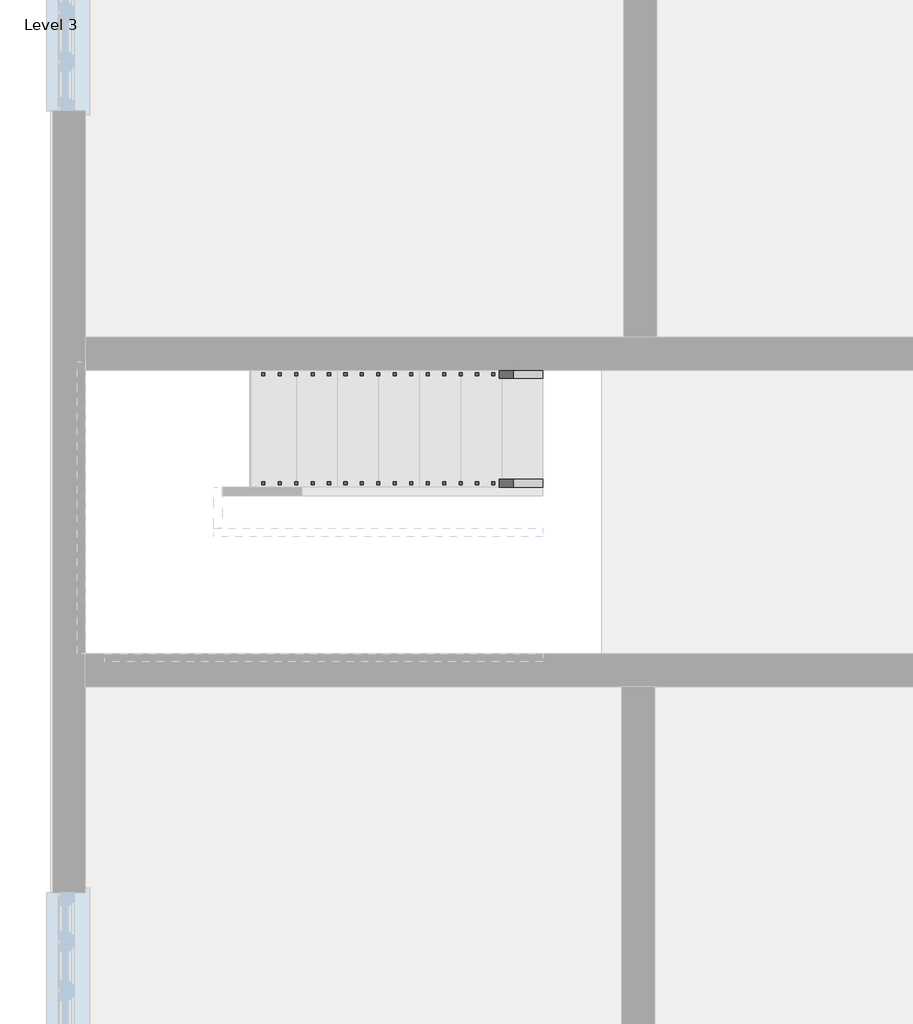
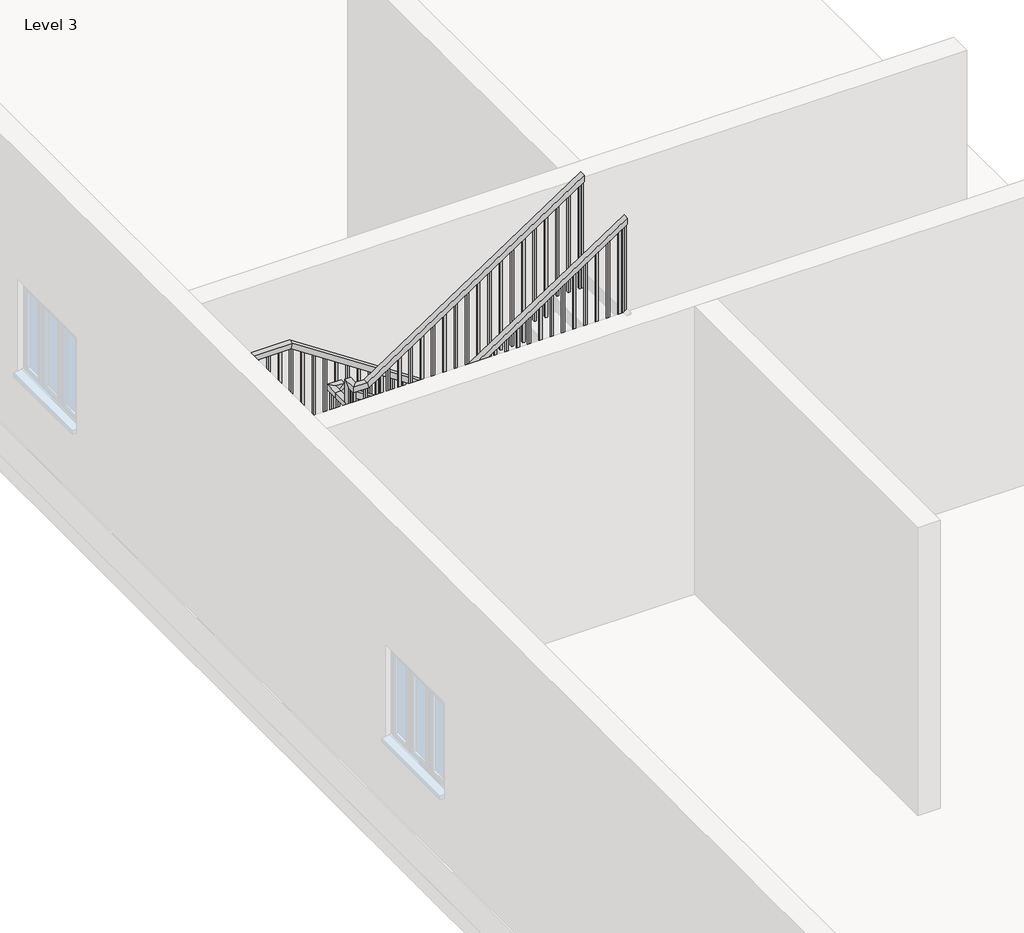
# One storey, part 2 of 3: 2 railings.
"""IFC4 building model written with IfcOpenShell, lengths in millimetres."""

from ifc_helpers import new_model, si_unit, frame, origin, place, context, project, spatial, polyline, outline, extrude, faceted_brep, element, save

model = new_model("IFC4")

# Units and contexts
model_context = context("Model", 3, world=origin())
ifc_project = project(units=[si_unit("LENGTHUNIT", "METRE", prefix="MILLI")], contexts=[model_context])

# Site, building, storey
site = spatial("IfcSite", under=ifc_project)
building = spatial("IfcBuilding", under=site)
storey = spatial("IfcBuildingStorey", under=building, Name="Level 3", Elevation=6096.0)

# Railings
placement = place(None, origin())
element("IfcRailing", 1, ObjectType="Handrail - Rectangular", at=placement, inside=storey, context=model_context, shape_type="SolidModel", body=[
    faceted_brep([(-2118.1728655, 1141.7797121, 7178.3222222), (-2118.1728655, 1141.7797121, 7117.4243166), (-2118.1728655, 1192.5797121, 7117.4243166), (-2118.1728655, 1192.5797121, 7178.3222222), (-4150.1728655, 1141.7797121, 8521.7), (-4165.4470084, 1141.7797121, 8470.9), (-4165.4470084, 1192.5797121, 8470.9), (-4150.1728655, 1192.5797121, 8521.7), (-4893.1394105, 1141.7797121, 8521.7), (-4893.1394105, 1141.7797121, 8470.9), (-4943.9394105, 1192.5797121, 8470.9), (-4943.9394105, 1192.5797121, 8521.7), (-4893.1394105, -509.2202879, 8521.7), (-4893.1394105, -509.2202879, 8470.9), (-4943.9394105, -560.0202879, 8470.9), (-4943.9394105, -560.0202879, 8521.7), (-4404.1728655, -509.2202879, 8521.7), (-4388.8987225, -509.2202879, 8470.9), (-4388.8987225, -560.0202879, 8470.9), (-4404.1728655, -560.0202879, 8521.7), (-2118.1728655, -509.2202879, 10033.0), (-2118.1728655, -560.0202879, 10033.0), (-2118.1728655, -560.0202879, 9972.1020944), (-2118.1728655, -509.2202879, 9972.1020944)], [[[0, 1, 2, 3]], [[1, 0, 4, 5]], [[2, 1, 5, 6]], [[3, 2, 6, 7]], [[0, 3, 7, 4]], [[5, 4, 8, 9]], [[6, 5, 9, 10]], [[7, 6, 10, 11]], [[4, 7, 11, 8]], [[9, 8, 12, 13]], [[10, 9, 13, 14]], [[11, 10, 14, 15]], [[8, 11, 15, 12]], [[13, 12, 16, 17]], [[14, 13, 17, 18]], [[15, 14, 18, 19]], [[12, 15, 19, 16]], [[20, 21, 22, 23]], [[17, 16, 20, 23]], [[18, 17, 23, 22]], [[19, 18, 22, 21]], [[16, 19, 21, 20]]]),
    extrude(outline(polyline([(9940.6057396, -2165.8144105), (9928.0115729, -2184.8644105), (8950.6777778, -2184.8644105), (8950.6777778, -2165.8144105), (9940.6057396, -2165.8144105)])), frame((0.0, -544.1452879, 0.0), z_axis=(0.0, 1.0, 0.0), x_axis=(0.0, 0.0, 1.0)), (0.0, 0.0, 1.0), 19.05),
    extrude(outline(polyline([(9873.4368507, -2267.4144105), (9860.842684, -2286.4644105), (8950.6777778, -2286.4644105), (8950.6777778, -2267.4144105), (9873.4368507, -2267.4144105)])), frame((0.0, -544.1452879, 0.0), z_axis=(0.0, 1.0, 0.0), x_axis=(0.0, 0.0, 1.0)), (0.0, 0.0, 1.0), 19.05),
    extrude(outline(polyline([(9806.2679618, -2369.0144105), (9793.6737951, -2388.0644105), (8782.7555556, -2388.0644105), (8782.7555556, -2369.0144105), (9806.2679618, -2369.0144105)])), frame((0.0, -544.1452879, 0.0), z_axis=(0.0, 1.0, 0.0), x_axis=(0.0, 0.0, 1.0)), (0.0, 0.0, 1.0), 19.05),
    extrude(outline(polyline([(9739.0990729, -2470.6144105), (9726.5049062, -2489.6644105), (8782.7555556, -2489.6644105), (8782.7555556, -2470.6144105), (9739.0990729, -2470.6144105)])), frame((0.0, -544.1452879, 0.0), z_axis=(0.0, 1.0, 0.0), x_axis=(0.0, 0.0, 1.0)), (0.0, 0.0, 1.0), 19.05),
    extrude(outline(polyline([(9671.930184, -2572.2144105), (9659.3360174, -2591.2644105), (8782.7555556, -2591.2644105), (8782.7555556, -2572.2144105), (9671.930184, -2572.2144105)])), frame((0.0, -544.1452879, 0.0), z_axis=(0.0, 1.0, 0.0), x_axis=(0.0, 0.0, 1.0)), (0.0, 0.0, 1.0), 19.05),
    extrude(outline(polyline([(9604.7612951, -2673.8144105), (9592.1671285, -2692.8644105), (8614.8333333, -2692.8644105), (8614.8333333, -2673.8144105), (9604.7612951, -2673.8144105)])), frame((0.0, -544.1452879, 0.0), z_axis=(0.0, 1.0, 0.0), x_axis=(0.0, 0.0, 1.0)), (0.0, 0.0, 1.0), 19.05),
    extrude(outline(polyline([(9537.5924062, -2775.4144105), (9524.9982396, -2794.4644105), (8614.8333333, -2794.4644105), (8614.8333333, -2775.4144105), (9537.5924062, -2775.4144105)])), frame((0.0, -544.1452879, 0.0), z_axis=(0.0, 1.0, 0.0), x_axis=(0.0, 0.0, 1.0)), (0.0, 0.0, 1.0), 19.05),
    extrude(outline(polyline([(9470.4235174, -2877.0144105), (9457.8293507, -2896.0644105), (8446.9111111, -2896.0644105), (8446.9111111, -2877.0144105), (9470.4235174, -2877.0144105)])), frame((0.0, -544.1452879, 0.0), z_axis=(0.0, 1.0, 0.0), x_axis=(0.0, 0.0, 1.0)), (0.0, 0.0, 1.0), 19.05),
    extrude(outline(polyline([(9403.2546285, -2978.6144105), (9390.6604618, -2997.6644105), (8446.9111111, -2997.6644105), (8446.9111111, -2978.6144105), (9403.2546285, -2978.6144105)])), frame((0.0, -544.1452879, 0.0), z_axis=(0.0, 1.0, 0.0), x_axis=(0.0, 0.0, 1.0)), (0.0, 0.0, 1.0), 19.05),
    extrude(outline(polyline([(9336.0857396, -3080.2144105), (9323.4915729, -3099.2644105), (8446.9111111, -3099.2644105), (8446.9111111, -3080.2144105), (9336.0857396, -3080.2144105)])), frame((0.0, -544.1452879, 0.0), z_axis=(0.0, 1.0, 0.0), x_axis=(0.0, 0.0, 1.0)), (0.0, 0.0, 1.0), 19.05),
    extrude(outline(polyline([(9268.9168507, -3181.8144105), (9256.322684, -3200.8644105), (8278.9888889, -3200.8644105), (8278.9888889, -3181.8144105), (9268.9168507, -3181.8144105)])), frame((0.0, -544.1452879, 0.0), z_axis=(0.0, 1.0, 0.0), x_axis=(0.0, 0.0, 1.0)), (0.0, 0.0, 1.0), 19.05),
    extrude(outline(polyline([(9201.7479618, -3283.4144105), (9189.1537951, -3302.4644105), (8278.9888889, -3302.4644105), (8278.9888889, -3283.4144105), (9201.7479618, -3283.4144105)])), frame((0.0, -544.1452879, 0.0), z_axis=(0.0, 1.0, 0.0), x_axis=(0.0, 0.0, 1.0)), (0.0, 0.0, 1.0), 19.05),
    extrude(outline(polyline([(9134.5790729, -3385.0144105), (9121.9849062, -3404.0644105), (8111.0666667, -3404.0644105), (8111.0666667, -3385.0144105), (9134.5790729, -3385.0144105)])), frame((0.0, -544.1452879, 0.0), z_axis=(0.0, 1.0, 0.0), x_axis=(0.0, 0.0, 1.0)), (0.0, 0.0, 1.0), 19.05),
    extrude(outline(polyline([(9067.410184, -3486.6144105), (9054.8160174, -3505.6644105), (8111.0666667, -3505.6644105), (8111.0666667, -3486.6144105), (9067.410184, -3486.6144105)])), frame((0.0, -544.1452879, 0.0), z_axis=(0.0, 1.0, 0.0), x_axis=(0.0, 0.0, 1.0)), (0.0, 0.0, 1.0), 19.05),
    extrude(outline(polyline([(9000.2412951, -3588.2144105), (8987.6471285, -3607.2644105), (8111.0666667, -3607.2644105), (8111.0666667, -3588.2144105), (9000.2412951, -3588.2144105)])), frame((0.0, -544.1452879, 0.0), z_axis=(0.0, 1.0, 0.0), x_axis=(0.0, 0.0, 1.0)), (0.0, 0.0, 1.0), 19.05),
    extrude(outline(polyline([(8933.0724062, -3689.8144105), (8920.4782396, -3708.8644105), (7943.1444444, -3708.8644105), (7943.1444444, -3689.8144105), (8933.0724062, -3689.8144105)])), frame((0.0, -544.1452879, 0.0), z_axis=(0.0, 1.0, 0.0), x_axis=(0.0, 0.0, 1.0)), (0.0, 0.0, 1.0), 19.05),
    extrude(outline(polyline([(8865.9035174, -3791.4144105), (8853.3093507, -3810.4644105), (7943.1444444, -3810.4644105), (7943.1444444, -3791.4144105), (8865.9035174, -3791.4144105)])), frame((0.0, -544.1452879, 0.0), z_axis=(0.0, 1.0, 0.0), x_axis=(0.0, 0.0, 1.0)), (0.0, 0.0, 1.0), 19.05),
    extrude(outline(polyline([(8798.7346285, -3893.0144105), (8786.1404618, -3912.0644105), (7775.2222222, -3912.0644105), (7775.2222222, -3893.0144105), (8798.7346285, -3893.0144105)])), frame((0.0, -544.1452879, 0.0), z_axis=(0.0, 1.0, 0.0), x_axis=(0.0, 0.0, 1.0)), (0.0, 0.0, 1.0), 19.05),
    extrude(outline(polyline([(8731.5657396, -3994.6144105), (8718.9715729, -4013.6644105), (7775.2222222, -4013.6644105), (7775.2222222, -3994.6144105), (8731.5657396, -3994.6144105)])), frame((0.0, -544.1452879, 0.0), z_axis=(0.0, 1.0, 0.0), x_axis=(0.0, 0.0, 1.0)), (0.0, 0.0, 1.0), 19.05),
    extrude(outline(polyline([(8664.3968507, -4096.2144105), (8651.802684, -4115.2644105), (7775.2222222, -4115.2644105), (7775.2222222, -4096.2144105), (8664.3968507, -4096.2144105)])), frame((0.0, -544.1452879, 0.0), z_axis=(0.0, 1.0, 0.0), x_axis=(0.0, 0.0, 1.0)), (0.0, 0.0, 1.0), 19.05),
    extrude(outline(polyline([(8597.2279618, -4197.8144105), (8584.6337951, -4216.8644105), (7607.3, -4216.8644105), (7607.3, -4197.8144105), (8597.2279618, -4197.8144105)])), frame((0.0, -544.1452879, 0.0), z_axis=(0.0, 1.0, 0.0), x_axis=(0.0, 0.0, 1.0)), (0.0, 0.0, 1.0), 19.05),
    extrude(outline(polyline([(8530.0590729, -4299.4144105), (8517.4649062, -4318.4644105), (7607.3, -4318.4644105), (7607.3, -4299.4144105), (8530.0590729, -4299.4144105)])), frame((0.0, -544.1452879, 0.0), z_axis=(0.0, 1.0, 0.0), x_axis=(0.0, 0.0, 1.0)), (0.0, 0.0, 1.0), 19.05),
    extrude(outline(polyline([(-4420.0644105, -544.1452879), (-4420.0644105, -525.0952879), (-4401.0144105, -525.0952879), (-4401.0144105, -544.1452879), (-4420.0644105, -544.1452879)])), frame((0.0, 0.0, 7607.3), z_axis=(0.0, 0.0, 1.0), x_axis=(1.0, 0.0, 0.0)), (0.0, 0.0, 1.0), 863.6),
    extrude(outline(polyline([(-4521.6644105, -544.1452879), (-4521.6644105, -525.0952879), (-4502.6144105, -525.0952879), (-4502.6144105, -544.1452879), (-4521.6644105, -544.1452879)])), frame((0.0, 0.0, 7607.3), z_axis=(0.0, 0.0, 1.0), x_axis=(1.0, 0.0, 0.0)), (0.0, 0.0, 1.0), 863.6),
    extrude(outline(polyline([(-4623.2644105, -544.1452879), (-4623.2644105, -525.0952879), (-4604.2144105, -525.0952879), (-4604.2144105, -544.1452879), (-4623.2644105, -544.1452879)])), frame((0.0, 0.0, 7607.3), z_axis=(0.0, 0.0, 1.0), x_axis=(1.0, 0.0, 0.0)), (0.0, 0.0, 1.0), 863.6),
    extrude(outline(polyline([(-4724.8644105, -544.1452879), (-4724.8644105, -525.0952879), (-4705.8144105, -525.0952879), (-4705.8144105, -544.1452879), (-4724.8644105, -544.1452879)])), frame((0.0, 0.0, 7607.3), z_axis=(0.0, 0.0, 1.0), x_axis=(1.0, 0.0, 0.0)), (0.0, 0.0, 1.0), 863.6),
    extrude(outline(polyline([(-4826.4644105, -544.1452879), (-4826.4644105, -525.0952879), (-4807.4144105, -525.0952879), (-4807.4144105, -544.1452879), (-4826.4644105, -544.1452879)])), frame((0.0, 0.0, 7607.3), z_axis=(0.0, 0.0, 1.0), x_axis=(1.0, 0.0, 0.0)), (0.0, 0.0, 1.0), 863.6),
    extrude(outline(polyline([(-4928.0644105, -448.8952879), (-4909.0144105, -448.8952879), (-4909.0144105, -467.9452879), (-4928.0644105, -467.9452879), (-4928.0644105, -448.8952879)])), frame((0.0, 0.0, 7607.3), z_axis=(0.0, 0.0, 1.0), x_axis=(1.0, 0.0, 0.0)), (0.0, 0.0, 1.0), 863.6),
    extrude(outline(polyline([(-4928.0644105, -347.2952879), (-4909.0144105, -347.2952879), (-4909.0144105, -366.3452879), (-4928.0644105, -366.3452879), (-4928.0644105, -347.2952879)])), frame((0.0, 0.0, 7607.3), z_axis=(0.0, 0.0, 1.0), x_axis=(1.0, 0.0, 0.0)), (0.0, 0.0, 1.0), 863.6),
    extrude(outline(polyline([(-4928.0644105, -245.6952879), (-4909.0144105, -245.6952879), (-4909.0144105, -264.7452879), (-4928.0644105, -264.7452879), (-4928.0644105, -245.6952879)])), frame((0.0, 0.0, 7607.3), z_axis=(0.0, 0.0, 1.0), x_axis=(1.0, 0.0, 0.0)), (0.0, 0.0, 1.0), 863.6),
    extrude(outline(polyline([(-4928.0644105, -144.0952879), (-4909.0144105, -144.0952879), (-4909.0144105, -163.1452879), (-4928.0644105, -163.1452879), (-4928.0644105, -144.0952879)])), frame((0.0, 0.0, 7607.3), z_axis=(0.0, 0.0, 1.0), x_axis=(1.0, 0.0, 0.0)), (0.0, 0.0, 1.0), 863.6),
    extrude(outline(polyline([(-4928.0644105, -42.4952879), (-4909.0144105, -42.4952879), (-4909.0144105, -61.5452879), (-4928.0644105, -61.5452879), (-4928.0644105, -42.4952879)])), frame((0.0, 0.0, 7607.3), z_axis=(0.0, 0.0, 1.0), x_axis=(1.0, 0.0, 0.0)), (0.0, 0.0, 1.0), 863.6),
    extrude(outline(polyline([(-4928.0644105, 59.1047121), (-4909.0144105, 59.1047121), (-4909.0144105, 40.0547121), (-4928.0644105, 40.0547121), (-4928.0644105, 59.1047121)])), frame((0.0, 0.0, 7607.3), z_axis=(0.0, 0.0, 1.0), x_axis=(1.0, 0.0, 0.0)), (0.0, 0.0, 1.0), 863.6),
    extrude(outline(polyline([(-4928.0644105, 160.7047121), (-4909.0144105, 160.7047121), (-4909.0144105, 141.6547121), (-4928.0644105, 141.6547121), (-4928.0644105, 160.7047121)])), frame((0.0, 0.0, 7607.3), z_axis=(0.0, 0.0, 1.0), x_axis=(1.0, 0.0, 0.0)), (0.0, 0.0, 1.0), 863.6),
    extrude(outline(polyline([(-4928.0644105, 262.3047121), (-4909.0144105, 262.3047121), (-4909.0144105, 243.2547121), (-4928.0644105, 243.2547121), (-4928.0644105, 262.3047121)])), frame((0.0, 0.0, 7607.3), z_axis=(0.0, 0.0, 1.0), x_axis=(1.0, 0.0, 0.0)), (0.0, 0.0, 1.0), 863.6),
    extrude(outline(polyline([(-4928.0644105, 363.9047121), (-4909.0144105, 363.9047121), (-4909.0144105, 344.8547121), (-4928.0644105, 344.8547121), (-4928.0644105, 363.9047121)])), frame((0.0, 0.0, 7607.3), z_axis=(0.0, 0.0, 1.0), x_axis=(1.0, 0.0, 0.0)), (0.0, 0.0, 1.0), 863.6),
    extrude(outline(polyline([(-4928.0644105, 465.5047121), (-4909.0144105, 465.5047121), (-4909.0144105, 446.4547121), (-4928.0644105, 446.4547121), (-4928.0644105, 465.5047121)])), frame((0.0, 0.0, 7607.3), z_axis=(0.0, 0.0, 1.0), x_axis=(1.0, 0.0, 0.0)), (0.0, 0.0, 1.0), 863.6),
    extrude(outline(polyline([(-4928.0644105, 567.1047121), (-4909.0144105, 567.1047121), (-4909.0144105, 548.0547121), (-4928.0644105, 548.0547121), (-4928.0644105, 567.1047121)])), frame((0.0, 0.0, 7607.3), z_axis=(0.0, 0.0, 1.0), x_axis=(1.0, 0.0, 0.0)), (0.0, 0.0, 1.0), 863.6),
    extrude(outline(polyline([(-4928.0644105, 668.7047121), (-4909.0144105, 668.7047121), (-4909.0144105, 649.6547121), (-4928.0644105, 649.6547121), (-4928.0644105, 668.7047121)])), frame((0.0, 0.0, 7607.3), z_axis=(0.0, 0.0, 1.0), x_axis=(1.0, 0.0, 0.0)), (0.0, 0.0, 1.0), 863.6),
    extrude(outline(polyline([(-4928.0644105, 770.3047121), (-4909.0144105, 770.3047121), (-4909.0144105, 751.2547121), (-4928.0644105, 751.2547121), (-4928.0644105, 770.3047121)])), frame((0.0, 0.0, 7607.3), z_axis=(0.0, 0.0, 1.0), x_axis=(1.0, 0.0, 0.0)), (0.0, 0.0, 1.0), 863.6),
    extrude(outline(polyline([(-4928.0644105, 871.9047121), (-4909.0144105, 871.9047121), (-4909.0144105, 852.8547121), (-4928.0644105, 852.8547121), (-4928.0644105, 871.9047121)])), frame((0.0, 0.0, 7607.3), z_axis=(0.0, 0.0, 1.0), x_axis=(1.0, 0.0, 0.0)), (0.0, 0.0, 1.0), 863.6),
    extrude(outline(polyline([(-4928.0644105, 973.5047121), (-4909.0144105, 973.5047121), (-4909.0144105, 954.4547121), (-4928.0644105, 954.4547121), (-4928.0644105, 973.5047121)])), frame((0.0, 0.0, 7607.3), z_axis=(0.0, 0.0, 1.0), x_axis=(1.0, 0.0, 0.0)), (0.0, 0.0, 1.0), 863.6),
    extrude(outline(polyline([(-4928.0644105, 1075.1047121), (-4909.0144105, 1075.1047121), (-4909.0144105, 1056.0547121), (-4928.0644105, 1056.0547121), (-4928.0644105, 1075.1047121)])), frame((0.0, 0.0, 7607.3), z_axis=(0.0, 0.0, 1.0), x_axis=(1.0, 0.0, 0.0)), (0.0, 0.0, 1.0), 863.6),
    extrude(outline(polyline([(-4851.8478655, 1176.7047121), (-4851.8478655, 1157.6547121), (-4870.8978655, 1157.6547121), (-4870.8978655, 1176.7047121), (-4851.8478655, 1176.7047121)])), frame((0.0, 0.0, 7607.3), z_axis=(0.0, 0.0, 1.0), x_axis=(1.0, 0.0, 0.0)), (0.0, 0.0, 1.0), 863.6),
    extrude(outline(polyline([(-4750.2478655, 1176.7047121), (-4750.2478655, 1157.6547121), (-4769.2978655, 1157.6547121), (-4769.2978655, 1176.7047121), (-4750.2478655, 1176.7047121)])), frame((0.0, 0.0, 7607.3), z_axis=(0.0, 0.0, 1.0), x_axis=(1.0, 0.0, 0.0)), (0.0, 0.0, 1.0), 863.6),
    extrude(outline(polyline([(-4648.6478655, 1176.7047121), (-4648.6478655, 1157.6547121), (-4667.6978655, 1157.6547121), (-4667.6978655, 1176.7047121), (-4648.6478655, 1176.7047121)])), frame((0.0, 0.0, 7607.3), z_axis=(0.0, 0.0, 1.0), x_axis=(1.0, 0.0, 0.0)), (0.0, 0.0, 1.0), 863.6),
    extrude(outline(polyline([(-4547.0478655, 1176.7047121), (-4547.0478655, 1157.6547121), (-4566.0978655, 1157.6547121), (-4566.0978655, 1176.7047121), (-4547.0478655, 1176.7047121)])), frame((0.0, 0.0, 7607.3), z_axis=(0.0, 0.0, 1.0), x_axis=(1.0, 0.0, 0.0)), (0.0, 0.0, 1.0), 863.6),
    extrude(outline(polyline([(-4445.4478655, 1176.7047121), (-4445.4478655, 1157.6547121), (-4464.4978655, 1157.6547121), (-4464.4978655, 1176.7047121), (-4445.4478655, 1176.7047121)])), frame((0.0, 0.0, 7607.3), z_axis=(0.0, 0.0, 1.0), x_axis=(1.0, 0.0, 0.0)), (0.0, 0.0, 1.0), 863.6),
    extrude(outline(polyline([(-4343.8478655, 1176.7047121), (-4343.8478655, 1157.6547121), (-4362.8978655, 1157.6547121), (-4362.8978655, 1176.7047121), (-4343.8478655, 1176.7047121)])), frame((0.0, 0.0, 7607.3), z_axis=(0.0, 0.0, 1.0), x_axis=(1.0, 0.0, 0.0)), (0.0, 0.0, 1.0), 863.6),
    extrude(outline(polyline([(-4242.2478655, 1176.7047121), (-4242.2478655, 1157.6547121), (-4261.2978655, 1157.6547121), (-4261.2978655, 1176.7047121), (-4242.2478655, 1176.7047121)])), frame((0.0, 0.0, 7607.3), z_axis=(0.0, 0.0, 1.0), x_axis=(1.0, 0.0, 0.0)), (0.0, 0.0, 1.0), 863.6),
    extrude(outline(polyline([(8454.505011, -4140.6478655), (8467.0991777, -4159.6978655), (7607.3, -4159.6978655), (7607.3, -4140.6478655), (8454.505011, -4140.6478655)])), frame((0.0, 1157.6547121, 0.0), z_axis=(0.0, 1.0, 0.0), x_axis=(0.0, 0.0, 1.0)), (0.0, 0.0, 1.0), 19.05),
    extrude(outline(polyline([(8387.3361222, -4039.0478655), (8399.9302888, -4058.0978655), (7439.3777778, -4058.0978655), (7439.3777778, -4039.0478655), (8387.3361222, -4039.0478655)])), frame((0.0, 1157.6547121, 0.0), z_axis=(0.0, 1.0, 0.0), x_axis=(0.0, 0.0, 1.0)), (0.0, 0.0, 1.0), 19.05),
    extrude(outline(polyline([(8320.1672333, -3937.4478655), (8332.7613999, -3956.4978655), (7439.3777778, -3956.4978655), (7439.3777778, -3937.4478655), (8320.1672333, -3937.4478655)])), frame((0.0, 1157.6547121, 0.0), z_axis=(0.0, 1.0, 0.0), x_axis=(0.0, 0.0, 1.0)), (0.0, 0.0, 1.0), 19.05),
    extrude(outline(polyline([(8252.9983444, -3835.8478655), (8265.592511, -3854.8978655), (7271.4555556, -3854.8978655), (7271.4555556, -3835.8478655), (8252.9983444, -3835.8478655)])), frame((0.0, 1157.6547121, 0.0), z_axis=(0.0, 1.0, 0.0), x_axis=(0.0, 0.0, 1.0)), (0.0, 0.0, 1.0), 19.05),
    extrude(outline(polyline([(8185.8294555, -3734.2478655), (8198.4236222, -3753.2978655), (7271.4555556, -3753.2978655), (7271.4555556, -3734.2478655), (8185.8294555, -3734.2478655)])), frame((0.0, 1157.6547121, 0.0), z_axis=(0.0, 1.0, 0.0), x_axis=(0.0, 0.0, 1.0)), (0.0, 0.0, 1.0), 19.05),
    extrude(outline(polyline([(8118.6605666, -3632.6478655), (8131.2547333, -3651.6978655), (7271.4555556, -3651.6978655), (7271.4555556, -3632.6478655), (8118.6605666, -3632.6478655)])), frame((0.0, 1157.6547121, 0.0), z_axis=(0.0, 1.0, 0.0), x_axis=(0.0, 0.0, 1.0)), (0.0, 0.0, 1.0), 19.05),
    extrude(outline(polyline([(8051.4916777, -3531.0478655), (8064.0858444, -3550.0978655), (7103.5333333, -3550.0978655), (7103.5333333, -3531.0478655), (8051.4916777, -3531.0478655)])), frame((0.0, 1157.6547121, 0.0), z_axis=(0.0, 1.0, 0.0), x_axis=(0.0, 0.0, 1.0)), (0.0, 0.0, 1.0), 19.05),
    extrude(outline(polyline([(7984.3227888, -3429.4478655), (7996.9169555, -3448.4978655), (7103.5333333, -3448.4978655), (7103.5333333, -3429.4478655), (7984.3227888, -3429.4478655)])), frame((0.0, 1157.6547121, 0.0), z_axis=(0.0, 1.0, 0.0), x_axis=(0.0, 0.0, 1.0)), (0.0, 0.0, 1.0), 19.05),
    extrude(outline(polyline([(7917.1538999, -3327.8478655), (7929.7480666, -3346.8978655), (6935.6111111, -3346.8978655), (6935.6111111, -3327.8478655), (7917.1538999, -3327.8478655)])), frame((0.0, 1157.6547121, 0.0), z_axis=(0.0, 1.0, 0.0), x_axis=(0.0, 0.0, 1.0)), (0.0, 0.0, 1.0), 19.05),
    extrude(outline(polyline([(7849.985011, -3226.2478655), (7862.5791777, -3245.2978655), (6935.6111111, -3245.2978655), (6935.6111111, -3226.2478655), (7849.985011, -3226.2478655)])), frame((0.0, 1157.6547121, 0.0), z_axis=(0.0, 1.0, 0.0), x_axis=(0.0, 0.0, 1.0)), (0.0, 0.0, 1.0), 19.05),
    extrude(outline(polyline([(7782.8161222, -3124.6478655), (7795.4102888, -3143.6978655), (6935.6111111, -3143.6978655), (6935.6111111, -3124.6478655), (7782.8161222, -3124.6478655)])), frame((0.0, 1157.6547121, 0.0), z_axis=(0.0, 1.0, 0.0), x_axis=(0.0, 0.0, 1.0)), (0.0, 0.0, 1.0), 19.05),
    extrude(outline(polyline([(7715.6472333, -3023.0478655), (7728.2413999, -3042.0978655), (6767.6888889, -3042.0978655), (6767.6888889, -3023.0478655), (7715.6472333, -3023.0478655)])), frame((0.0, 1157.6547121, 0.0), z_axis=(0.0, 1.0, 0.0), x_axis=(0.0, 0.0, 1.0)), (0.0, 0.0, 1.0), 19.05),
    extrude(outline(polyline([(7648.4783444, -2921.4478655), (7661.072511, -2940.4978655), (6767.6888889, -2940.4978655), (6767.6888889, -2921.4478655), (7648.4783444, -2921.4478655)])), frame((0.0, 1157.6547121, 0.0), z_axis=(0.0, 1.0, 0.0), x_axis=(0.0, 0.0, 1.0)), (0.0, 0.0, 1.0), 19.05),
    extrude(outline(polyline([(7581.3094555, -2819.8478655), (7593.9036222, -2838.8978655), (6599.7666667, -2838.8978655), (6599.7666667, -2819.8478655), (7581.3094555, -2819.8478655)])), frame((0.0, 1157.6547121, 0.0), z_axis=(0.0, 1.0, 0.0), x_axis=(0.0, 0.0, 1.0)), (0.0, 0.0, 1.0), 19.05),
    extrude(outline(polyline([(7514.1405666, -2718.2478655), (7526.7347333, -2737.2978655), (6599.7666667, -2737.2978655), (6599.7666667, -2718.2478655), (7514.1405666, -2718.2478655)])), frame((0.0, 1157.6547121, 0.0), z_axis=(0.0, 1.0, 0.0), x_axis=(0.0, 0.0, 1.0)), (0.0, 0.0, 1.0), 19.05),
    extrude(outline(polyline([(7446.9716777, -2616.6478655), (7459.5658444, -2635.6978655), (6599.7666667, -2635.6978655), (6599.7666667, -2616.6478655), (7446.9716777, -2616.6478655)])), frame((0.0, 1157.6547121, 0.0), z_axis=(0.0, 1.0, 0.0), x_axis=(0.0, 0.0, 1.0)), (0.0, 0.0, 1.0), 19.05),
    extrude(outline(polyline([(7379.8027888, -2515.0478655), (7392.3969555, -2534.0978655), (6431.8444444, -2534.0978655), (6431.8444444, -2515.0478655), (7379.8027888, -2515.0478655)])), frame((0.0, 1157.6547121, 0.0), z_axis=(0.0, 1.0, 0.0), x_axis=(0.0, 0.0, 1.0)), (0.0, 0.0, 1.0), 19.05),
    extrude(outline(polyline([(7312.6338999, -2413.4478655), (7325.2280666, -2432.4978655), (6431.8444444, -2432.4978655), (6431.8444444, -2413.4478655), (7312.6338999, -2413.4478655)])), frame((0.0, 1157.6547121, 0.0), z_axis=(0.0, 1.0, 0.0), x_axis=(0.0, 0.0, 1.0)), (0.0, 0.0, 1.0), 19.05),
    extrude(outline(polyline([(7245.465011, -2311.8478655), (7258.0591777, -2330.8978655), (6263.9222222, -2330.8978655), (6263.9222222, -2311.8478655), (7245.465011, -2311.8478655)])), frame((0.0, 1157.6547121, 0.0), z_axis=(0.0, 1.0, 0.0), x_axis=(0.0, 0.0, 1.0)), (0.0, 0.0, 1.0), 19.05),
    extrude(outline(polyline([(7178.2961222, -2210.2478655), (7190.8902888, -2229.2978655), (6263.9222222, -2229.2978655), (6263.9222222, -2210.2478655), (7178.2961222, -2210.2478655)])), frame((0.0, 1157.6547121, 0.0), z_axis=(0.0, 1.0, 0.0), x_axis=(0.0, 0.0, 1.0)), (0.0, 0.0, 1.0), 19.05),
    extrude(outline(polyline([(-4928.0644105, -525.0952879), (-4909.0144105, -525.0952879), (-4909.0144105, -544.1452879), (-4928.0644105, -544.1452879), (-4928.0644105, -525.0952879)])), frame((0.0, 0.0, 7607.3), z_axis=(0.0, 0.0, 1.0), x_axis=(1.0, 0.0, 0.0)), (0.0, 0.0, 1.0), 863.6),
    extrude(outline(polyline([(-4909.0144105, 1176.7047121), (-4909.0144105, 1157.6547121), (-4928.0644105, 1157.6547121), (-4928.0644105, 1176.7047121), (-4909.0144105, 1176.7047121)])), frame((0.0, 0.0, 7607.3), z_axis=(0.0, 0.0, 1.0), x_axis=(1.0, 0.0, 0.0)), (0.0, 0.0, 1.0), 863.6),
    extrude(outline(polyline([(9972.1020944, -2118.1728655), (9959.5079277, -2137.2228655), (8950.6777778, -2137.2228655), (8950.6777778, -2118.1728655), (9972.1020944, -2118.1728655)])), frame((0.0, -544.1452879, 0.0), z_axis=(0.0, 1.0, 0.0), x_axis=(0.0, 0.0, 1.0)), (0.0, 0.0, 1.0), 19.05),
    extrude(outline(polyline([(7117.4243166, -2118.1728655), (7130.0184833, -2137.2228655), (6263.9222222, -2137.2228655), (6263.9222222, -2118.1728655), (7117.4243166, -2118.1728655)])), frame((0.0, 1157.6547121, 0.0), z_axis=(0.0, 1.0, 0.0), x_axis=(0.0, 0.0, 1.0)), (0.0, 0.0, 1.0), 19.05),
])
element("IfcRailing", 2, ObjectType="Handrail - Rectangular", at=placement, inside=storey, context=model_context, shape_type="SolidModel", body=[
    faceted_brep([(-2118.1728655, 468.6797121, 7178.3222222), (-2118.1728655, 468.6797121, 7117.4243166), (-2118.1728655, 519.4797121, 7117.4243166), (-2118.1728655, 519.4797121, 7178.3222222), (-4073.9728655, 468.6797121, 8471.3233333), (-4124.7728655, 468.6797121, 8444.0098722), (-4124.7728655, 519.4797121, 8444.0098722), (-4073.9728655, 519.4797121, 8471.3233333), (-4073.9728655, 468.6797121, 8521.7), (-4124.7728655, 468.6797121, 8470.9), (-4124.7728655, 519.4797121, 8470.9), (-4073.9728655, 519.4797121, 8521.7), (-4150.1728655, 468.6797121, 8521.7), (-4150.1728655, 468.6797121, 8470.9), (-4200.9728655, 519.4797121, 8470.9), (-4200.9728655, 519.4797121, 8521.7), (-4150.1728655, 392.4797121, 8521.7), (-4150.1728655, 392.4797121, 8470.9), (-4200.9728655, 392.4797121, 8470.9), (-4200.9728655, 392.4797121, 8521.7), (-4150.1728655, 240.0797121, 8521.7), (-4150.1728655, 189.2797121, 8470.9), (-4200.9728655, 189.2797121, 8470.9), (-4200.9728655, 240.0797121, 8521.7), (-4150.1728655, 240.0797121, 8739.9988889), (-4150.1728655, 189.2797121, 8689.1988889), (-4200.9728655, 189.2797121, 8689.1988889), (-4200.9728655, 240.0797121, 8739.9988889), (-4150.1728655, 163.8797121, 8739.9988889), (-4150.1728655, 163.8797121, 8689.1988889), (-4200.9728655, 113.0797121, 8689.1988889), (-4200.9728655, 113.0797121, 8739.9988889), (-4073.9728655, 163.8797121, 8739.9988889), (-4058.6987225, 163.8797121, 8689.1988889), (-4058.6987225, 113.0797121, 8689.1988889), (-4073.9728655, 113.0797121, 8739.9988889), (-2118.1728655, 163.8797121, 10033.0), (-2118.1728655, 113.0797121, 10033.0), (-2118.1728655, 113.0797121, 9972.1020944), (-2118.1728655, 163.8797121, 9972.1020944)], [[[0, 1, 2, 3]], [[1, 0, 4, 5]], [[2, 1, 5, 6]], [[3, 2, 6, 7]], [[0, 3, 7, 4]], [[5, 4, 8, 9]], [[6, 5, 9, 10]], [[7, 6, 10, 11]], [[4, 7, 11, 8]], [[9, 8, 12, 13]], [[10, 9, 13, 14]], [[11, 10, 14, 15]], [[8, 11, 15, 12]], [[13, 12, 16, 17]], [[14, 13, 17, 18]], [[15, 14, 18, 19]], [[12, 15, 19, 16]], [[17, 16, 20, 21]], [[18, 17, 21, 22]], [[19, 18, 22, 23]], [[16, 19, 23, 20]], [[21, 20, 24, 25]], [[22, 21, 25, 26]], [[23, 22, 26, 27]], [[20, 23, 27, 24]], [[25, 24, 28, 29]], [[26, 25, 29, 30]], [[27, 26, 30, 31]], [[24, 27, 31, 28]], [[29, 28, 32, 33]], [[30, 29, 33, 34]], [[31, 30, 34, 35]], [[28, 31, 35, 32]], [[36, 37, 38, 39]], [[33, 32, 36, 39]], [[34, 33, 39, 38]], [[35, 34, 38, 37]], [[32, 35, 37, 36]]]),
    extrude(outline(polyline([(9949.0127888, -2153.0978655), (8950.6777778, -2153.0978655), (8950.6777778, -2134.0478655), (9961.6069555, -2134.0478655), (9949.0127888, -2153.0978655)])), frame((0.0, 128.9547121, 0.0), z_axis=(0.0, 1.0, 0.0), x_axis=(0.0, 0.0, 1.0)), (0.0, 0.0, 1.0), 19.05),
    extrude(outline(polyline([(9881.8438999, -2254.6978655), (8950.6777778, -2254.6978655), (8950.6777778, -2235.6478655), (9894.4380666, -2235.6478655), (9881.8438999, -2254.6978655)])), frame((0.0, 128.9547121, 0.0), z_axis=(0.0, 1.0, 0.0), x_axis=(0.0, 0.0, 1.0)), (0.0, 0.0, 1.0), 19.05),
    extrude(outline(polyline([(9814.675011, -2356.2978655), (8950.6777778, -2356.2978655), (8950.6777778, -2337.2478655), (9827.2691777, -2337.2478655), (9814.675011, -2356.2978655)])), frame((0.0, 128.9547121, 0.0), z_axis=(0.0, 1.0, 0.0), x_axis=(0.0, 0.0, 1.0)), (0.0, 0.0, 1.0), 19.05),
    extrude(outline(polyline([(9747.5061222, -2457.8978655), (8782.7555556, -2457.8978655), (8782.7555556, -2438.8478655), (9760.1002888, -2438.8478655), (9747.5061222, -2457.8978655)])), frame((0.0, 128.9547121, 0.0), z_axis=(0.0, 1.0, 0.0), x_axis=(0.0, 0.0, 1.0)), (0.0, 0.0, 1.0), 19.05),
    extrude(outline(polyline([(9680.3372333, -2559.4978655), (8782.7555556, -2559.4978655), (8782.7555556, -2540.4478655), (9692.9313999, -2540.4478655), (9680.3372333, -2559.4978655)])), frame((0.0, 128.9547121, 0.0), z_axis=(0.0, 1.0, 0.0), x_axis=(0.0, 0.0, 1.0)), (0.0, 0.0, 1.0), 19.05),
    extrude(outline(polyline([(9613.1683444, -2661.0978655), (8614.8333333, -2661.0978655), (8614.8333333, -2642.0478655), (9625.762511, -2642.0478655), (9613.1683444, -2661.0978655)])), frame((0.0, 128.9547121, 0.0), z_axis=(0.0, 1.0, 0.0), x_axis=(0.0, 0.0, 1.0)), (0.0, 0.0, 1.0), 19.05),
    extrude(outline(polyline([(9545.9994555, -2762.6978655), (8614.8333333, -2762.6978655), (8614.8333333, -2743.6478655), (9558.5936222, -2743.6478655), (9545.9994555, -2762.6978655)])), frame((0.0, 128.9547121, 0.0), z_axis=(0.0, 1.0, 0.0), x_axis=(0.0, 0.0, 1.0)), (0.0, 0.0, 1.0), 19.05),
    extrude(outline(polyline([(9478.8305666, -2864.2978655), (8614.8333333, -2864.2978655), (8614.8333333, -2845.2478655), (9491.4247333, -2845.2478655), (9478.8305666, -2864.2978655)])), frame((0.0, 128.9547121, 0.0), z_axis=(0.0, 1.0, 0.0), x_axis=(0.0, 0.0, 1.0)), (0.0, 0.0, 1.0), 19.05),
    extrude(outline(polyline([(9411.6616777, -2965.8978655), (8446.9111111, -2965.8978655), (8446.9111111, -2946.8478655), (9424.2558444, -2946.8478655), (9411.6616777, -2965.8978655)])), frame((0.0, 128.9547121, 0.0), z_axis=(0.0, 1.0, 0.0), x_axis=(0.0, 0.0, 1.0)), (0.0, 0.0, 1.0), 19.05),
    extrude(outline(polyline([(9344.4927888, -3067.4978655), (8446.9111111, -3067.4978655), (8446.9111111, -3048.4478655), (9357.0869555, -3048.4478655), (9344.4927888, -3067.4978655)])), frame((0.0, 128.9547121, 0.0), z_axis=(0.0, 1.0, 0.0), x_axis=(0.0, 0.0, 1.0)), (0.0, 0.0, 1.0), 19.05),
    extrude(outline(polyline([(9277.3238999, -3169.0978655), (8278.9888889, -3169.0978655), (8278.9888889, -3150.0478655), (9289.9180666, -3150.0478655), (9277.3238999, -3169.0978655)])), frame((0.0, 128.9547121, 0.0), z_axis=(0.0, 1.0, 0.0), x_axis=(0.0, 0.0, 1.0)), (0.0, 0.0, 1.0), 19.05),
    extrude(outline(polyline([(9210.155011, -3270.6978655), (8278.9888889, -3270.6978655), (8278.9888889, -3251.6478655), (9222.7491777, -3251.6478655), (9210.155011, -3270.6978655)])), frame((0.0, 128.9547121, 0.0), z_axis=(0.0, 1.0, 0.0), x_axis=(0.0, 0.0, 1.0)), (0.0, 0.0, 1.0), 19.05),
    extrude(outline(polyline([(9142.9861222, -3372.2978655), (8278.9888889, -3372.2978655), (8278.9888889, -3353.2478655), (9155.5802888, -3353.2478655), (9142.9861222, -3372.2978655)])), frame((0.0, 128.9547121, 0.0), z_axis=(0.0, 1.0, 0.0), x_axis=(0.0, 0.0, 1.0)), (0.0, 0.0, 1.0), 19.05),
    extrude(outline(polyline([(9075.8172333, -3473.8978655), (8111.0666667, -3473.8978655), (8111.0666667, -3454.8478655), (9088.4113999, -3454.8478655), (9075.8172333, -3473.8978655)])), frame((0.0, 128.9547121, 0.0), z_axis=(0.0, 1.0, 0.0), x_axis=(0.0, 0.0, 1.0)), (0.0, 0.0, 1.0), 19.05),
    extrude(outline(polyline([(9008.6483444, -3575.4978655), (8111.0666667, -3575.4978655), (8111.0666667, -3556.4478655), (9021.242511, -3556.4478655), (9008.6483444, -3575.4978655)])), frame((0.0, 128.9547121, 0.0), z_axis=(0.0, 1.0, 0.0), x_axis=(0.0, 0.0, 1.0)), (0.0, 0.0, 1.0), 19.05),
    extrude(outline(polyline([(8941.4794555, -3677.0978655), (7943.1444444, -3677.0978655), (7943.1444444, -3658.0478655), (8954.0736222, -3658.0478655), (8941.4794555, -3677.0978655)])), frame((0.0, 128.9547121, 0.0), z_axis=(0.0, 1.0, 0.0), x_axis=(0.0, 0.0, 1.0)), (0.0, 0.0, 1.0), 19.05),
    extrude(outline(polyline([(8874.3105666, -3778.6978655), (7943.1444444, -3778.6978655), (7943.1444444, -3759.6478655), (8886.9047333, -3759.6478655), (8874.3105666, -3778.6978655)])), frame((0.0, 128.9547121, 0.0), z_axis=(0.0, 1.0, 0.0), x_axis=(0.0, 0.0, 1.0)), (0.0, 0.0, 1.0), 19.05),
    extrude(outline(polyline([(8807.1416777, -3880.2978655), (7943.1444444, -3880.2978655), (7943.1444444, -3861.2478655), (8819.7358444, -3861.2478655), (8807.1416777, -3880.2978655)])), frame((0.0, 128.9547121, 0.0), z_axis=(0.0, 1.0, 0.0), x_axis=(0.0, 0.0, 1.0)), (0.0, 0.0, 1.0), 19.05),
    extrude(outline(polyline([(8739.9727888, -3981.8978655), (7775.2222222, -3981.8978655), (7775.2222222, -3962.8478655), (8752.5669555, -3962.8478655), (8739.9727888, -3981.8978655)])), frame((0.0, 128.9547121, 0.0), z_axis=(0.0, 1.0, 0.0), x_axis=(0.0, 0.0, 1.0)), (0.0, 0.0, 1.0), 19.05),
    extrude(outline(polyline([(8672.8038999, -4083.4978655), (7775.2222222, -4083.4978655), (7775.2222222, -4064.4478655), (8685.3980666, -4064.4478655), (8672.8038999, -4083.4978655)])), frame((0.0, 128.9547121, 0.0), z_axis=(0.0, 1.0, 0.0), x_axis=(0.0, 0.0, 1.0)), (0.0, 0.0, 1.0), 19.05),
    extrude(outline(polyline([(-4166.0478655, 198.8047121), (-4166.0478655, 179.7547121), (-4185.0978655, 179.7547121), (-4185.0978655, 198.8047121), (-4166.0478655, 198.8047121)])), frame((0.0, 0.0, 7607.3), z_axis=(0.0, 0.0, 1.0), x_axis=(1.0, 0.0, 0.0)), (0.0, 0.0, 1.0), 1081.8988889),
    extrude(outline(polyline([(-4166.0478655, 300.4047121), (-4166.0478655, 281.3547121), (-4185.0978655, 281.3547121), (-4185.0978655, 300.4047121), (-4166.0478655, 300.4047121)])), frame((0.0, 0.0, 7607.3), z_axis=(0.0, 0.0, 1.0), x_axis=(1.0, 0.0, 0.0)), (0.0, 0.0, 1.0), 863.6),
    extrude(outline(polyline([(-4166.0478655, 402.0047121), (-4166.0478655, 382.9547121), (-4185.0978655, 382.9547121), (-4185.0978655, 402.0047121), (-4166.0478655, 402.0047121)])), frame((0.0, 0.0, 7607.3), z_axis=(0.0, 0.0, 1.0), x_axis=(1.0, 0.0, 0.0)), (0.0, 0.0, 1.0), 863.6),
    extrude(outline(polyline([(-4140.6478655, 484.5547121), (-4159.6978655, 484.5547121), (-4159.6978655, 503.6047121), (-4140.6478655, 503.6047121), (-4140.6478655, 484.5547121)])), frame((0.0, 0.0, 7607.3), z_axis=(0.0, 0.0, 1.0), x_axis=(1.0, 0.0, 0.0)), (0.0, 0.0, 1.0), 863.6),
    extrude(outline(polyline([(8399.9302888, -4058.0978655), (7439.3777778, -4058.0978655), (7439.3777778, -4039.0478655), (8387.3361222, -4039.0478655), (8399.9302888, -4058.0978655)])), frame((0.0, 484.5547121, 0.0), z_axis=(0.0, 1.0, 0.0), x_axis=(0.0, 0.0, 1.0)), (0.0, 0.0, 1.0), 19.05),
    extrude(outline(polyline([(8332.7613999, -3956.4978655), (7439.3777778, -3956.4978655), (7439.3777778, -3937.4478655), (8320.1672333, -3937.4478655), (8332.7613999, -3956.4978655)])), frame((0.0, 484.5547121, 0.0), z_axis=(0.0, 1.0, 0.0), x_axis=(0.0, 0.0, 1.0)), (0.0, 0.0, 1.0), 19.05),
    extrude(outline(polyline([(8265.592511, -3854.8978655), (7271.4555556, -3854.8978655), (7271.4555556, -3835.8478655), (8252.9983444, -3835.8478655), (8265.592511, -3854.8978655)])), frame((0.0, 484.5547121, 0.0), z_axis=(0.0, 1.0, 0.0), x_axis=(0.0, 0.0, 1.0)), (0.0, 0.0, 1.0), 19.05),
    extrude(outline(polyline([(8198.4236222, -3753.2978655), (7271.4555556, -3753.2978655), (7271.4555556, -3734.2478655), (8185.8294555, -3734.2478655), (8198.4236222, -3753.2978655)])), frame((0.0, 484.5547121, 0.0), z_axis=(0.0, 1.0, 0.0), x_axis=(0.0, 0.0, 1.0)), (0.0, 0.0, 1.0), 19.05),
    extrude(outline(polyline([(8131.2547333, -3651.6978655), (7271.4555556, -3651.6978655), (7271.4555556, -3632.6478655), (8118.6605666, -3632.6478655), (8131.2547333, -3651.6978655)])), frame((0.0, 484.5547121, 0.0), z_axis=(0.0, 1.0, 0.0), x_axis=(0.0, 0.0, 1.0)), (0.0, 0.0, 1.0), 19.05),
    extrude(outline(polyline([(8064.0858444, -3550.0978655), (7103.5333333, -3550.0978655), (7103.5333333, -3531.0478655), (8051.4916777, -3531.0478655), (8064.0858444, -3550.0978655)])), frame((0.0, 484.5547121, 0.0), z_axis=(0.0, 1.0, 0.0), x_axis=(0.0, 0.0, 1.0)), (0.0, 0.0, 1.0), 19.05),
    extrude(outline(polyline([(7996.9169555, -3448.4978655), (7103.5333333, -3448.4978655), (7103.5333333, -3429.4478655), (7984.3227888, -3429.4478655), (7996.9169555, -3448.4978655)])), frame((0.0, 484.5547121, 0.0), z_axis=(0.0, 1.0, 0.0), x_axis=(0.0, 0.0, 1.0)), (0.0, 0.0, 1.0), 19.05),
    extrude(outline(polyline([(7929.7480666, -3346.8978655), (6935.6111111, -3346.8978655), (6935.6111111, -3327.8478655), (7917.1538999, -3327.8478655), (7929.7480666, -3346.8978655)])), frame((0.0, 484.5547121, 0.0), z_axis=(0.0, 1.0, 0.0), x_axis=(0.0, 0.0, 1.0)), (0.0, 0.0, 1.0), 19.05),
    extrude(outline(polyline([(7862.5791777, -3245.2978655), (6935.6111111, -3245.2978655), (6935.6111111, -3226.2478655), (7849.985011, -3226.2478655), (7862.5791777, -3245.2978655)])), frame((0.0, 484.5547121, 0.0), z_axis=(0.0, 1.0, 0.0), x_axis=(0.0, 0.0, 1.0)), (0.0, 0.0, 1.0), 19.05),
    extrude(outline(polyline([(7795.4102888, -3143.6978655), (6935.6111111, -3143.6978655), (6935.6111111, -3124.6478655), (7782.8161222, -3124.6478655), (7795.4102888, -3143.6978655)])), frame((0.0, 484.5547121, 0.0), z_axis=(0.0, 1.0, 0.0), x_axis=(0.0, 0.0, 1.0)), (0.0, 0.0, 1.0), 19.05),
    extrude(outline(polyline([(7728.2413999, -3042.0978655), (6767.6888889, -3042.0978655), (6767.6888889, -3023.0478655), (7715.6472333, -3023.0478655), (7728.2413999, -3042.0978655)])), frame((0.0, 484.5547121, 0.0), z_axis=(0.0, 1.0, 0.0), x_axis=(0.0, 0.0, 1.0)), (0.0, 0.0, 1.0), 19.05),
    extrude(outline(polyline([(7661.072511, -2940.4978655), (6767.6888889, -2940.4978655), (6767.6888889, -2921.4478655), (7648.4783444, -2921.4478655), (7661.072511, -2940.4978655)])), frame((0.0, 484.5547121, 0.0), z_axis=(0.0, 1.0, 0.0), x_axis=(0.0, 0.0, 1.0)), (0.0, 0.0, 1.0), 19.05),
    extrude(outline(polyline([(7593.9036222, -2838.8978655), (6599.7666667, -2838.8978655), (6599.7666667, -2819.8478655), (7581.3094555, -2819.8478655), (7593.9036222, -2838.8978655)])), frame((0.0, 484.5547121, 0.0), z_axis=(0.0, 1.0, 0.0), x_axis=(0.0, 0.0, 1.0)), (0.0, 0.0, 1.0), 19.05),
    extrude(outline(polyline([(7526.7347333, -2737.2978655), (6599.7666667, -2737.2978655), (6599.7666667, -2718.2478655), (7514.1405666, -2718.2478655), (7526.7347333, -2737.2978655)])), frame((0.0, 484.5547121, 0.0), z_axis=(0.0, 1.0, 0.0), x_axis=(0.0, 0.0, 1.0)), (0.0, 0.0, 1.0), 19.05),
    extrude(outline(polyline([(7459.5658444, -2635.6978655), (6599.7666667, -2635.6978655), (6599.7666667, -2616.6478655), (7446.9716777, -2616.6478655), (7459.5658444, -2635.6978655)])), frame((0.0, 484.5547121, 0.0), z_axis=(0.0, 1.0, 0.0), x_axis=(0.0, 0.0, 1.0)), (0.0, 0.0, 1.0), 19.05),
    extrude(outline(polyline([(7392.3969555, -2534.0978655), (6431.8444444, -2534.0978655), (6431.8444444, -2515.0478655), (7379.8027888, -2515.0478655), (7392.3969555, -2534.0978655)])), frame((0.0, 484.5547121, 0.0), z_axis=(0.0, 1.0, 0.0), x_axis=(0.0, 0.0, 1.0)), (0.0, 0.0, 1.0), 19.05),
    extrude(outline(polyline([(7325.2280666, -2432.4978655), (6431.8444444, -2432.4978655), (6431.8444444, -2413.4478655), (7312.6338999, -2413.4478655), (7325.2280666, -2432.4978655)])), frame((0.0, 484.5547121, 0.0), z_axis=(0.0, 1.0, 0.0), x_axis=(0.0, 0.0, 1.0)), (0.0, 0.0, 1.0), 19.05),
    extrude(outline(polyline([(7258.0591777, -2330.8978655), (6263.9222222, -2330.8978655), (6263.9222222, -2311.8478655), (7245.465011, -2311.8478655), (7258.0591777, -2330.8978655)])), frame((0.0, 484.5547121, 0.0), z_axis=(0.0, 1.0, 0.0), x_axis=(0.0, 0.0, 1.0)), (0.0, 0.0, 1.0), 19.05),
    extrude(outline(polyline([(7190.8902888, -2229.2978655), (6263.9222222, -2229.2978655), (6263.9222222, -2210.2478655), (7178.2961222, -2210.2478655), (7190.8902888, -2229.2978655)])), frame((0.0, 484.5547121, 0.0), z_axis=(0.0, 1.0, 0.0), x_axis=(0.0, 0.0, 1.0)), (0.0, 0.0, 1.0), 19.05),
    extrude(outline(polyline([(-4166.0478655, 148.0047121), (-4166.0478655, 128.9547121), (-4185.0978655, 128.9547121), (-4185.0978655, 148.0047121), (-4166.0478655, 148.0047121)])), frame((0.0, 0.0, 7607.3), z_axis=(0.0, 0.0, 1.0), x_axis=(1.0, 0.0, 0.0)), (0.0, 0.0, 1.0), 1081.8988889),
    extrude(outline(polyline([(-4166.0478655, 484.5547121), (-4185.0978655, 484.5547121), (-4185.0978655, 503.6047121), (-4166.0478655, 503.6047121), (-4166.0478655, 484.5547121)])), frame((0.0, 0.0, 7607.3), z_axis=(0.0, 0.0, 1.0), x_axis=(1.0, 0.0, 0.0)), (0.0, 0.0, 1.0), 863.6),
    extrude(outline(polyline([(9959.5079277, -2137.2228655), (8950.6777778, -2137.2228655), (8950.6777778, -2118.1728655), (9972.1020944, -2118.1728655), (9959.5079277, -2137.2228655)])), frame((0.0, 128.9547121, 0.0), z_axis=(0.0, 1.0, 0.0), x_axis=(0.0, 0.0, 1.0)), (0.0, 0.0, 1.0), 19.05),
    extrude(outline(polyline([(7130.0184833, -2137.2228655), (6263.9222222, -2137.2228655), (6263.9222222, -2118.1728655), (7117.4243166, -2118.1728655), (7130.0184833, -2137.2228655)])), frame((0.0, 484.5547121, 0.0), z_axis=(0.0, 1.0, 0.0), x_axis=(0.0, 0.0, 1.0)), (0.0, 0.0, 1.0), 19.05),
])

save(model, "model.ifc")

# Revit data of these elements
# Type "Handrail - Rectangular"
#   Assembly Code = "C2010400"
#   built-in parameter 1008612 = 0.0416667 (stored number, unit not read)
#   built-in parameter 1008611 = 0.0416667 (stored number, unit not read)
#   built-in parameter 1008609 = 0.333333 (stored number, unit not read)
#   built-in parameter 1008604 = 0.166667 (stored number, unit not read)
#   built-in parameter 1008603 = 0.166667 (stored number, unit not read)
#   Railing Height = 914.4 mm
#   built-in parameter 1008630 = 2
#   built-in parameter 1008610 = 2
#   built-in parameter 1008618 = Baluster - Square : 3/4"
# Elements 1, 2 (IfcRailing, "Handrail - Rectangular")
#   Phase Created = New Construction
